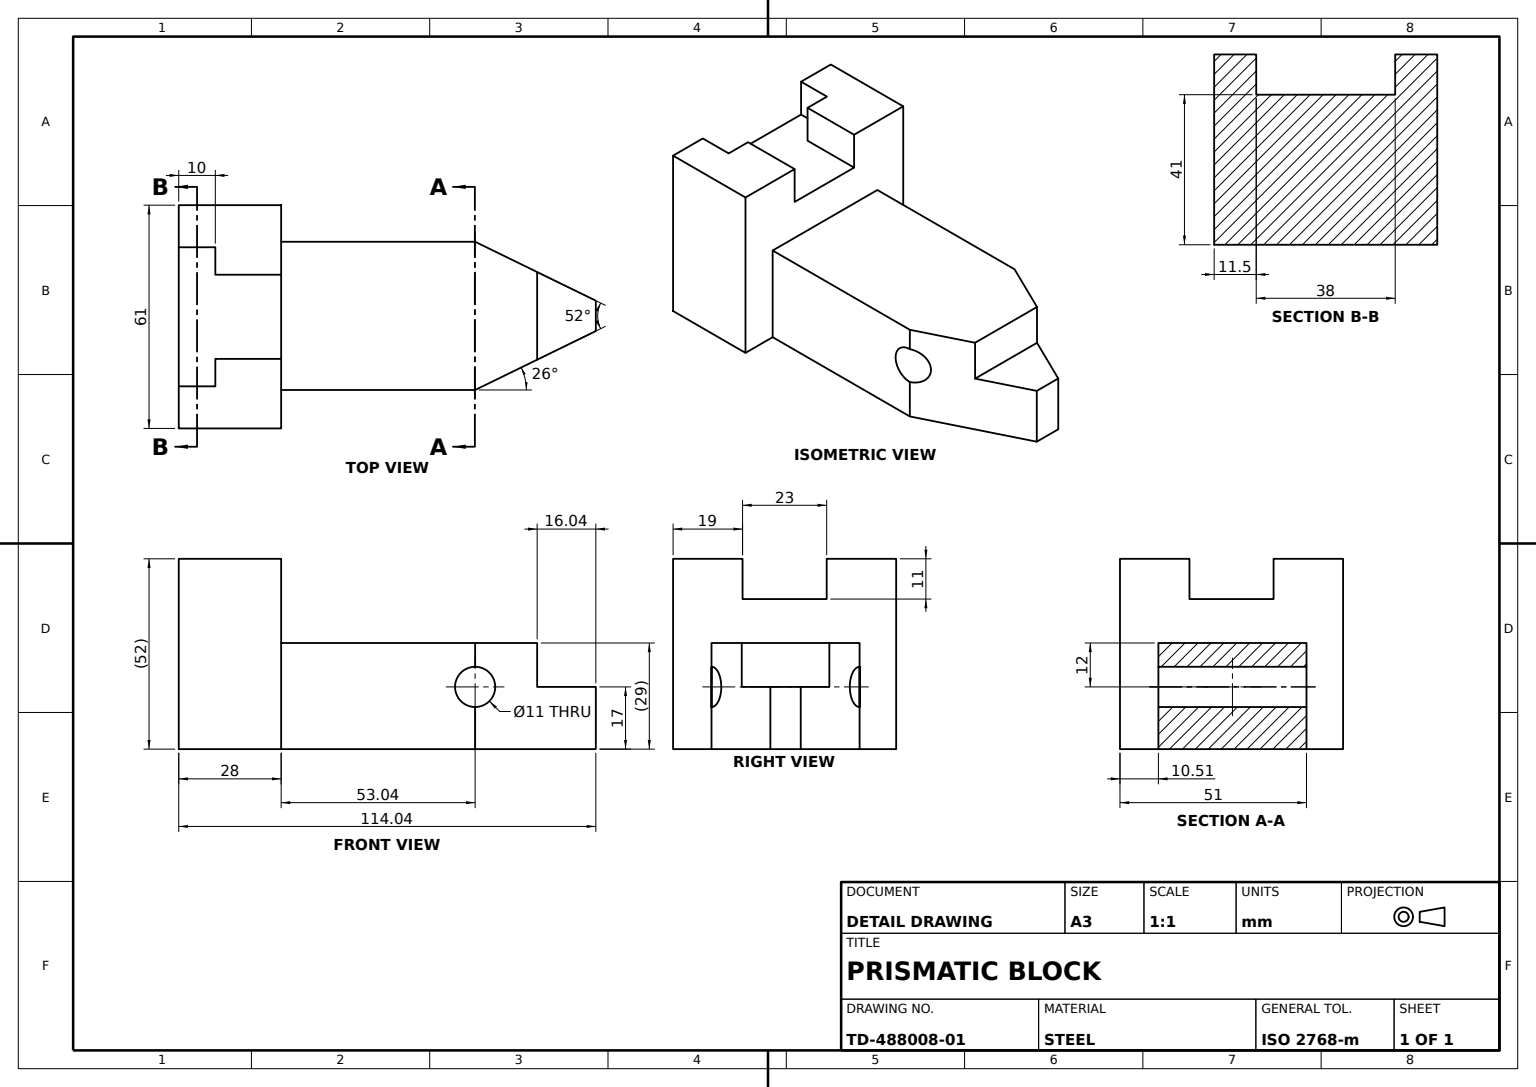
from build123d import *

# Parameters (mm, degrees)
BASE_BLOCK_PROFILE_W         = 61
BASE_BLOCK_PROFILE_H         = 41
BASE_BLOCK_41X61X120_DEPTH   = 120
LENGTHWISE_STEP_CUT_DEPTH    = 120
CASTELLATED_END_BOSSES_DEPTH = 11
TAPERED_NOSE_CUT_DEPTH       = 128.759539761
TAPERED_NOSE_CUT_DEPTH_BACK  = 51
TAPERED_NOSE_PROFILE_W       = 10
TAPERED_NOSE_PROFILE_H       = 86.04422701
TAPERED_NOSE_PROFILE_W_2     = 10.506122453
NOSE_SLOT_CUT_DEPTH          = 51
CROSS_HOLE_DEPTH             = 128.759539761
CROSS_HOLE_DEPTH_BACK        = 128.759539761
CROSS_HOLE_PROFILE_R         = 5.5


with BuildPart() as part:
    # Base Block Profile → Base Block 41x61x120 (new body)
    with BuildSketch(Plane.XY):
        Rectangle(BASE_BLOCK_PROFILE_W, BASE_BLOCK_PROFILE_H)
    extrude(amount=BASE_BLOCK_41X61X120_DEPTH)

    # Step Cut Profile → Lengthwise Step Cut (cut)
    with BuildSketch(Plane(origin=(30.5, 0, 0), x_dir=(0, 0, -1), z_dir=(1, 0, 0))):
        Polygon((-22, -3.5), (0, -3.5), (0, 20.5), (-92, 20.5), (-92, 8.5), (-22, 8.5), align=None)
    extrude(amount=-LENGTHWISE_STEP_CUT_DEPTH, mode=Mode.SUBTRACT)

    # End Boss Profile → Castellated End Bosses (add)
    with BuildSketch(Plane(origin=(0, 20.5, 0), x_dir=(1, 0, 0), z_dir=(0, 1, 0))):
        Polygon((-19, -120), (-30.5, -120), (-30.5, -92), (-11.5, -92), (-11.5, -110), (-19, -110), align=None)
        Polygon((11.5, -92), (30.5, -92), (30.5, -120), (19, -120), (19, -110), (11.5, -110), align=None)
    extrude(amount=CASTELLATED_END_BOSSES_DEPTH)

    # Tapered Nose Profile → Tapered Nose Cut (cut, two sides: drawn at the far end of the back side and taken through both)
    with BuildSketch(Plane(origin=(0, 0, 0), x_dir=(1, 0, 0), z_dir=(0, 1, 0)).offset(-TAPERED_NOSE_CUT_DEPTH_BACK)):
        with Locations((-25.5, -48.977886495)):
            Rectangle(TAPERED_NOSE_PROFILE_W, TAPERED_NOSE_PROFILE_H)
        with Locations((25.246938774, -48.977886495)):
            Rectangle(TAPERED_NOSE_PROFILE_W_2, TAPERED_NOSE_PROFILE_H)
        Polygon((19.993877547, -5.95577299), (3.898702125, -5.95577299), (19.993877547, -38.95577299), align=None)
        Polygon((-20.5, -38.95577299), (-4.404824577, -5.95577299), (-20.5, -5.95577299), align=None)
    extrude(amount=TAPERED_NOSE_CUT_DEPTH + TAPERED_NOSE_CUT_DEPTH_BACK, mode=Mode.SUBTRACT)

    # Nose Slot Profile → Nose Slot Cut (cut)
    with BuildSketch(Plane(origin=(0, -3.5, 0), x_dir=(1, 0, 0), z_dir=(0, 1, 0))):
        Polygon((-30.5, -5.95577299), (3.898702125, -5.95577299), (30.5, -5.95577299), (30.5, 0), (-30.5, 0), align=None)
    extrude(amount=-NOSE_SLOT_CUT_DEPTH, mode=Mode.SUBTRACT)

    # Cross Hole Profile → Cross Hole (cut, two sides: drawn at the far end of the back side and taken through both)
    with BuildSketch(Plane(origin=(0, 0, 0), x_dir=(0, 0, -1), z_dir=(1, 0, 0)).offset(-CROSS_HOLE_DEPTH_BACK)):
        with Locations(Location((-38.95577299, -3.5, 0), (0, 0, 90))):
            Circle(CROSS_HOLE_PROFILE_R)
    extrude(amount=CROSS_HOLE_DEPTH + CROSS_HOLE_DEPTH_BACK, mode=Mode.SUBTRACT)


solid = part.part
